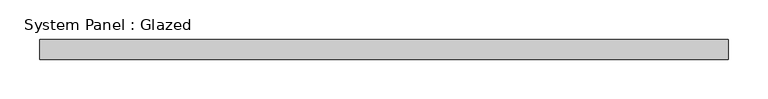
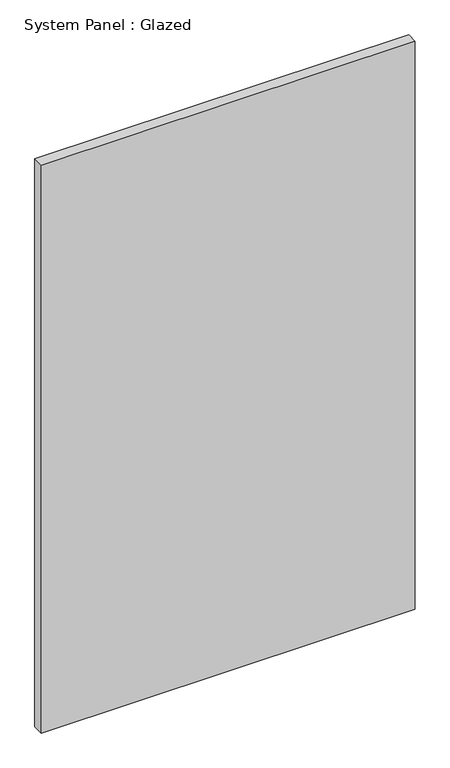
"""IFC4 building model written with IfcOpenShell, lengths in millimetres: plate geometry, System Panel : Glazed."""

from ifc_helpers import new_model, si_unit, origin, origin_with_axes, place, context, project, spatial, polyline, outline, extrude, source, transform, mapped, element, save


def system_panel_glazed_4c7522cd(model_context):
    return source(origin(), model_context, "Body", "SweptSolid", [
        extrude(outline(polyline([(434.975, 19.05), (-434.975, 19.05), (-434.975, 44.45), (434.975, 44.45), (434.975, 19.05)])), origin_with_axes(), (0.0, 0.0, 1.0), 1396.1033231),
    ])


if __name__ == "__main__":
    model = new_model("IFC4")
    model_context = context("Model", 3, world=origin())
    ifc_project = project(units=[si_unit("LENGTHUNIT", "METRE", prefix="MILLI")], contexts=[model_context])
    site = spatial("IfcSite", under=ifc_project)
    building = spatial("IfcBuilding", under=site)
    placement = place(None, origin())
    system_panel_glazed_shape = system_panel_glazed_4c7522cd(model_context)
    element("IfcPlate", 1, ObjectType="System Panel : Glazed", at=placement, inside=building, context=model_context, shape_type="MappedRepresentation", body=[
        mapped(system_panel_glazed_shape, transform((0.0, 0.0, 0.0), x_axis=(1.0, 0.0, 0.0), y_axis=(0.0, 1.0, 0.0), z_axis=(0.0, 0.0, 1.0))),
    ])
    save(model, "model.ifc")

# Revit data of these elements
# Type "System Panel : Glazed"
#   Construction Type Id = "GSP4R"
#   Analytic Construction = "1/8 in Pilkington single glazing"
#   Visual Light Transmittance = 0.9
#   Solar Heat Gain Coefficient = 0.86
#   Heat Transfer Coefficient (U) = 1.18115 BTU/(h·ft²·°F)
#   Define Thermal Properties by = 1
# Element 1 (IfcPlate, "System Panel : Glazed")
#   Materials on its faces: "Glass"
# Materials
#   "Glass": class "Glass", colour RGB 0 128 192, transparency 0.75, Description = "Soda Lime Glass", Cost = 0
